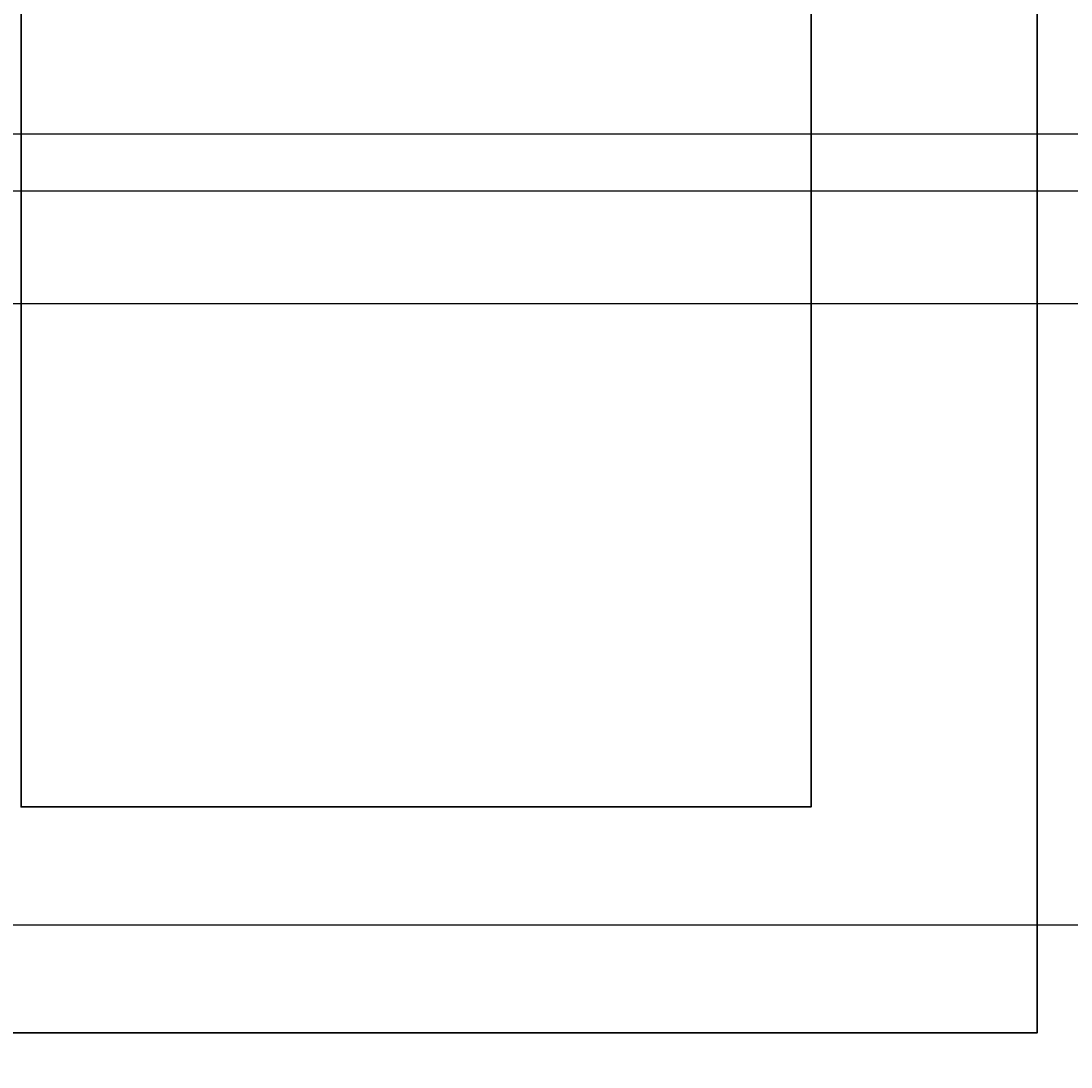
# Model space of a CAD drawing. Units: inches. Extents: x -6 to 289, y -8 to 323.
# Tile 13 of 107: x 46 to 102, y 68 to 124. Entities that reach past the tile are written whole.
import ezdxf

# ---------------------------------------------------------------- set-up
doc = ezdxf.new("R2010")
doc.units = ezdxf.units.IN
doc.header["$MEASUREMENT"] = 0
doc.layers.add('A-ANNO-DIMS', color=2, linetype='Continuous', lineweight=18)
doc.layers.add('A-ELEV', color=7, linetype='Continuous', lineweight=35)
doc.styles.get("Standard").update_dxf_attribs({"font": 'arial.ttf'})
doc.dimstyles.get("Standard").update_dxf_attribs({"dimtxt": 0.18, "dimasz": 0.18, "dimexe": 0.18, "dimexo": 0.0625, "dimgap": 0.09, "dimtad": 0, "dimtih": 1, "dimtoh": 1, "dimdec": 4, "dimzin": 0, "dimdsep": 46, "dimtxsty": 'Standard', "dimcen": 0.09, "dimadec": 0, "dimazin": 0, "dimtfac": 1, "dimtdec": 4, "dimtofl": 0, "dimtmove": 0, "dimatfit": 3, "dimfxl": 1, "dimtolj": 1, "dimtzin": 0, "dimarcsym": 0})

# ---------------------------------------------------------------- blocks, each defined once
blk = doc.blocks.new('*D86')
at = {"layer": 'A-ANNO-DIMS', "color": 0, "lineweight": -2, "transparency": 16777216}
for p, q in [((166.233, 75.971), (-5.737, 75.971)), ((-5.557, 75.791), (-5.557, 63.71)), ((-5.557, 51.265), (-5.557, 63.346)), ((120.945, 51.085), (-5.737, 51.085))]:
    blk.add_line(p, q, dxfattribs=at)
at = {"layer": 'A-ANNO-DIMS', "color": 0, "transparency": 16777216}
for points in [[(-5.587, 75.791), (-5.527, 75.791), (-5.557, 75.971)], [(-5.587, 51.265), (-5.527, 51.265), (-5.557, 51.085)]]:
    blk.add_solid(points, dxfattribs=at)
at = {"layer": 'Defpoints', "color": 0, "transparency": 16777216}
for p in [(-5.557, 75.971), (166.296, 75.971), (121.008, 51.085)]:
    blk.add_point(p, dxfattribs=at)
at = {"layer": 'A-ANNO-DIMS', "color": 0, "transparency": 16777216, "insert": (-5.557, 63.528), "char_height": 0.18, "attachment_point": 5}
blk.add_mtext('\\A1;24.886', dxfattribs=at)
blk = doc.blocks.new('*D87')
at = {"layer": 'A-ANNO-DIMS', "color": 0, "lineweight": -2, "transparency": 16777216}
for p, q in [((142.233, 108.948), (-5.737, 108.948)), ((-5.557, 108.768), (-5.557, 92.641)), ((-5.557, 76.151), (-5.557, 92.277)), ((166.233, 75.971), (-5.737, 75.971))]:
    blk.add_line(p, q, dxfattribs=at)
at = {"layer": 'A-ANNO-DIMS', "color": 0, "transparency": 16777216}
for points in [[(-5.587, 108.768), (-5.527, 108.768), (-5.557, 108.948)], [(-5.587, 76.151), (-5.527, 76.151), (-5.557, 75.971)]]:
    blk.add_solid(points, dxfattribs=at)
at = {"layer": 'Defpoints', "color": 0, "transparency": 16777216}
for p in [(-5.557, 108.948), (142.296, 108.948), (166.296, 75.971)]:
    blk.add_point(p, dxfattribs=at)
at = {"layer": 'A-ANNO-DIMS', "color": 0, "transparency": 16777216, "insert": (-5.557, 92.459), "char_height": 0.18, "attachment_point": 5}
blk.add_mtext('\\A1;32.98', dxfattribs=at)
blk = doc.blocks.new('*D88')
at = {"layer": 'A-ANNO-DIMS', "color": 0, "lineweight": -2, "transparency": 16777216}
for p, q in [((138.233, 114.948), (-5.737, 114.948)), ((-5.557, 114.768), (-5.557, 112.13)), ((-5.557, 109.128), (-5.557, 111.766)), ((142.233, 108.948), (-5.737, 108.948))]:
    blk.add_line(p, q, dxfattribs=at)
at = {"layer": 'A-ANNO-DIMS', "color": 0, "transparency": 16777216}
for points in [[(-5.587, 114.768), (-5.527, 114.768), (-5.557, 114.948)], [(-5.587, 109.128), (-5.527, 109.128), (-5.557, 108.948)]]:
    blk.add_solid(points, dxfattribs=at)
at = {"layer": 'Defpoints', "color": 0, "transparency": 16777216}
for p in [(-5.557, 114.948), (138.296, 114.948), (142.296, 108.948)]:
    blk.add_point(p, dxfattribs=at)
at = {"layer": 'A-ANNO-DIMS', "color": 0, "transparency": 16777216, "insert": (-5.557, 111.948), "char_height": 0.18, "attachment_point": 5}
blk.add_mtext('\\A1;6', dxfattribs=at)
blk = doc.blocks.new('*D89')
at = {"layer": 'A-ANNO-DIMS', "color": 0, "lineweight": -2, "transparency": 16777216}
for p, q in [((135.233, 117.971), (-5.737, 117.971)), ((-5.557, 117.791), (-5.557, 116.641)), ((-5.557, 115.128), (-5.557, 116.277)), ((138.233, 114.948), (-5.737, 114.948))]:
    blk.add_line(p, q, dxfattribs=at)
at = {"layer": 'A-ANNO-DIMS', "color": 0, "transparency": 16777216}
for points in [[(-5.587, 117.791), (-5.527, 117.791), (-5.557, 117.971)], [(-5.587, 115.128), (-5.527, 115.128), (-5.557, 114.948)]]:
    blk.add_solid(points, dxfattribs=at)
at = {"layer": 'Defpoints', "color": 0, "transparency": 16777216}
for p in [(-5.557, 117.971), (135.296, 117.971), (138.296, 114.948)]:
    blk.add_point(p, dxfattribs=at)
at = {"layer": 'A-ANNO-DIMS', "color": 0, "transparency": 16777216, "insert": (-5.557, 116.459), "char_height": 0.18, "attachment_point": 5}
blk.add_mtext('\\A1;3.023', dxfattribs=at)

msp = doc.modelspace()

# ---------------------------------------------------------------- linework, layer by layer
at = {"layer": 'A-ELEV'}
for points in [[(33.7437, 289.0427), (99.7007, 289.0427), (99.7007, 70.2425), (33.7437, 70.2425)], [(45.7437, 277.0427), (87.7007, 277.0427), (87.7007, 82.2425), (45.7437, 82.2425)]]:
    msp.add_lwpolyline(points, close=True, dxfattribs=at)

# ---------------------------------------------------------------- dimensions: what is measured, and where the dimension line sits
at = {"layer": 'A-ANNO-DIMS'}
for base, p1, p2, override, picture, middle in [((-5.557, 117.9706), (138.296, 114.9477), (135.296, 117.9706), {"dimdec": 3, "dimlfac": 1, "dimrnd": 0, "dimzin": 0, "dimdsep": 46, "dimlunit": 2}, '*D89', (-5.557, 116.4592)), ((-5.557, 114.9477), (142.296, 108.9477), (138.296, 114.9477), {"dimdec": 0, "dimlfac": 1, "dimrnd": 0, "dimzin": 0, "dimdsep": 46, "dimlunit": 2}, '*D88', (-5.557, 111.9477)), ((-5.557, 108.9477), (166.296, 75.9706), (142.296, 108.9477), {"dimdec": 2, "dimlfac": 1, "dimrnd": 0, "dimzin": 0, "dimdsep": 46, "dimlunit": 2}, '*D87', (-5.557, 92.4592)), ((-5.557, 75.97064), (121.00798, 51.08513), (166.29599, 75.97064), {"dimdec": 3, "dimlfac": 1, "dimrnd": 0, "dimzin": 0, "dimdsep": 46, "dimlunit": 2}, '*D86', (-5.557, 63.52788))]:
    dim = msp.add_linear_dim(base=base, p1=p1, p2=p2, angle=90, dimstyle='Standard', override=override, dxfattribs=at)
    dim.commit()
    dim.dimension.update_dxf_attribs({"geometry": picture, "text_midpoint": middle})

doc.saveas('drawing.dxf')
